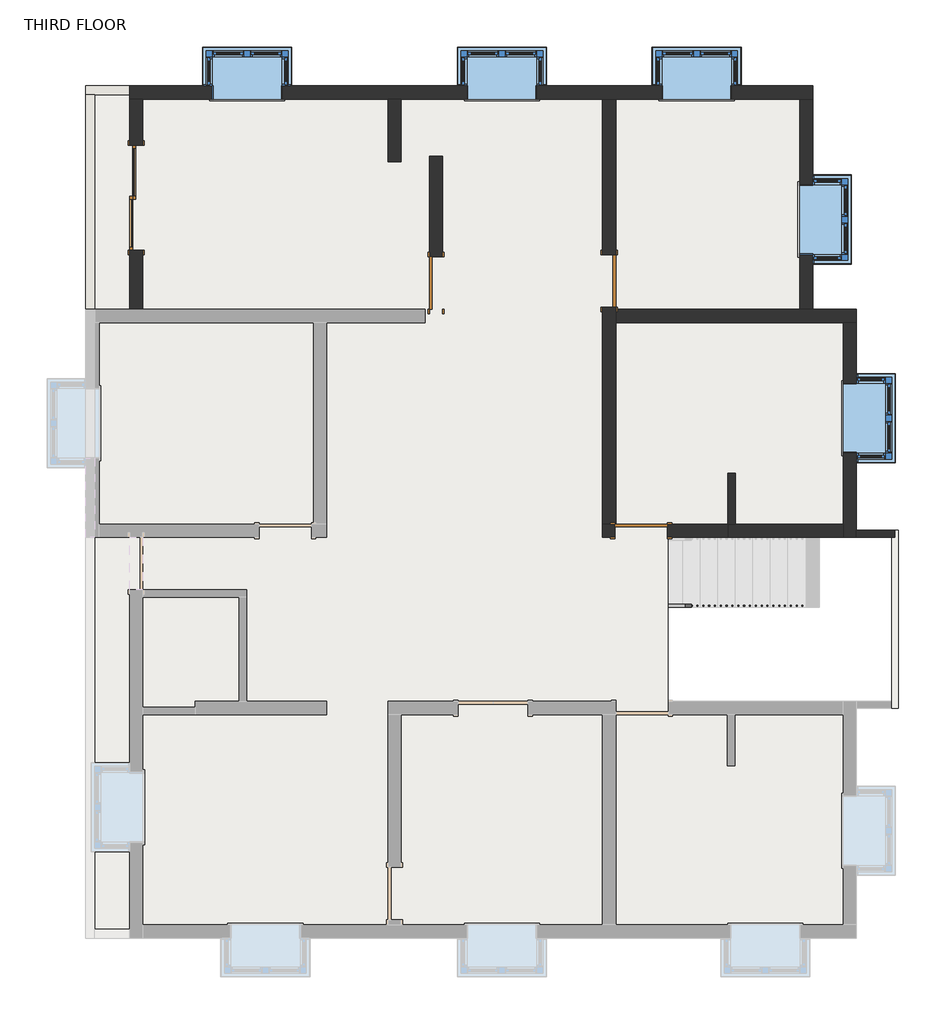
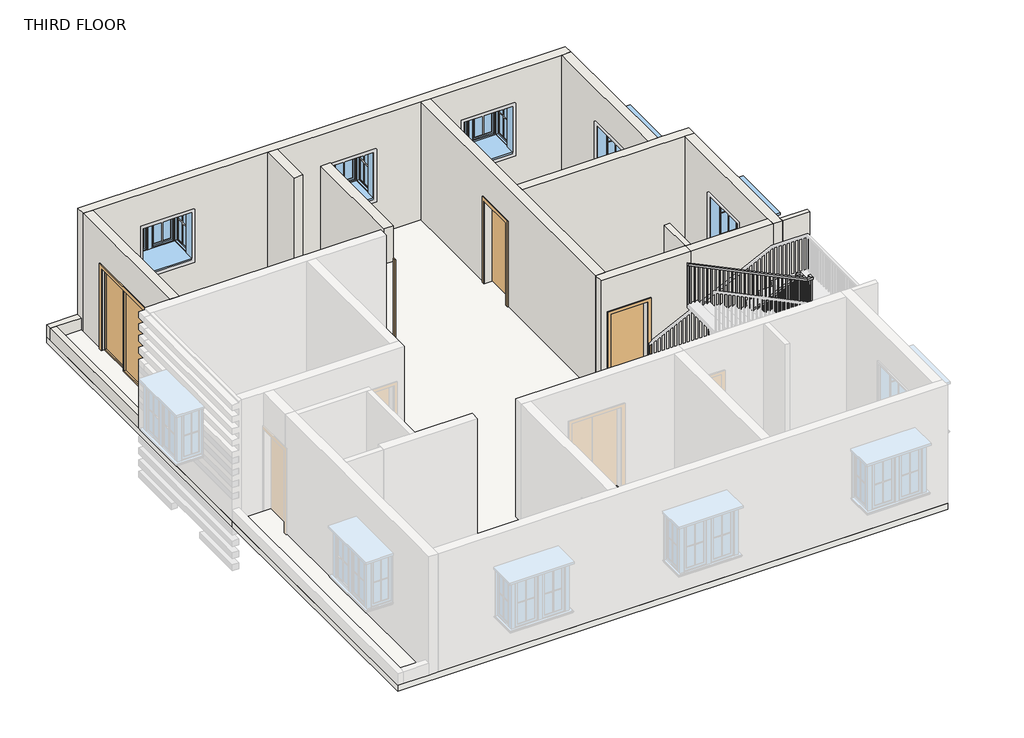
# One storey, part 2 of 4: 14 walls, 5 windows, 4 doors, 1 railing, 1 slab.
"""IFC4 building model written with IfcOpenShell, lengths in millimetres."""

from ifc_helpers import new_model, si_unit, frame, origin, place, context, project, spatial, polyline, outline, extrude, faceted_brep, transform, mapped, element, save
from components import door_d4d75d1e, door_a90ba1ad, door_0ca8825f, window_bay_casement_box_90_degree_angle_4_x4_x2_07b705a1

model = new_model("IFC4")

# Units and contexts
model_context = context("Model", 3, world=origin())
ifc_project = project(units=[si_unit("LENGTHUNIT", "METRE", prefix="MILLI")], contexts=[model_context])

# Site, building, storey
site = spatial("IfcSite", under=ifc_project)
building = spatial("IfcBuilding", under=site)
storey = spatial("IfcBuildingStorey", under=building, Name="THIRD FLOOR", Elevation=9601.2)

# Doors
placement = place(None, origin())
door_shape = door_d4d75d1e(model_context)
element("IfcDoor", 1, ObjectType="Door-Double-Sliding : 72\" x 84\"", at=placement, inside=storey, context=model_context, shape_type="MappedRepresentation", body=[
    mapped(door_shape, transform((-6005.0415084, 6126.233346, 9601.2), x_axis=(0.0, 1.0, 0.0), y_axis=(-1.0, 0.0, 0.0), z_axis=(0.0, 0.0, 1.0))),
])
door_2_shape = door_a90ba1ad(model_context)
element("IfcDoor", 2, ObjectType="Single-Flush : 36\" x 84\"", at=placement, inside=storey, context=model_context, shape_type="MappedRepresentation", body=[
    mapped(door_2_shape, transform((2656.3584916, 335.033346, 9601.2), x_axis=(-1.0, 0.0, 0.0), y_axis=(0.0, -1.0, 0.0), z_axis=(0.0, 0.0, 1.0))),
])
element("IfcDoor", 3, ObjectType="Single-Flush : 36\" x 84\"", at=placement, inside=storey, context=model_context, shape_type="MappedRepresentation", body=[
    mapped(door_2_shape, transform((-918.5024437, 4640.333346, 9601.2), x_axis=(0.0, -1.0, 0.0), y_axis=(1.0, 0.0, 0.0), z_axis=(0.0, 0.0, 1.0))),
])
door_3_shape = door_0ca8825f(model_context)
element("IfcDoor", 4, ObjectType="Single-Flush : 36\" x 84\"", at=placement, inside=storey, context=model_context, shape_type="MappedRepresentation", body=[
    mapped(door_3_shape, transform((2097.5584916, 4678.433346, 9601.2), x_axis=(0.0, -1.0, 0.0), y_axis=(1.0, 0.0, 0.0), z_axis=(0.0, 0.0, 1.0))),
])

# Railing
element("IfcRailing", 5, ObjectType="Handrail - Rectangular", at=placement, inside=storey, context=model_context, shape_type="SolidModel", body=[
    faceted_brep([(3126.2584916, -947.666654, 10661.0727273), (3126.2584916, -947.666654, 10604.5956113), (3126.2584916, -998.466654, 10604.5956113), (3126.2584916, -998.466654, 10661.0727273), (6044.5829507, -947.666654, 12078.7823634), (6095.3829507, -947.666654, 12046.9836718), (6095.3829507, -998.466654, 12046.9836718), (6044.5829507, -998.466654, 12078.7823634), (6044.5829507, -947.666654, 12115.8), (6095.3829507, -947.666654, 12065.0), (6095.3829507, -998.466654, 12065.0), (6044.5829507, -998.466654, 12115.8), (6171.5829507, -947.666654, 12115.8), (6171.5829507, -947.666654, 12065.0), (6120.7829507, -998.466654, 12065.0), (6120.7829507, -998.466654, 12115.8), (6171.5829507, -1074.666654, 12115.8), (6171.5829507, -1074.666654, 12065.0), (6120.7829507, -1074.666654, 12065.0), (6120.7829507, -1074.666654, 12115.8), (6171.5829507, -1341.366654, 12115.8), (6171.5829507, -1392.166654, 12065.0), (6120.7829507, -1392.166654, 12065.0), (6120.7829507, -1341.366654, 12115.8), (6171.5829507, -1341.366654, 12298.2903639), (6171.5829507, -1392.166654, 12247.4903639), (6120.7829507, -1392.166654, 12247.4903639), (6120.7829507, -1341.366654, 12298.2903639), (6171.5829507, -1468.366654, 12298.2903639), (6171.5829507, -1468.366654, 12247.4903639), (6120.7829507, -1417.566654, 12247.4903639), (6120.7829507, -1417.566654, 12298.2903639), (6044.5829507, -1468.366654, 12298.2903639), (6032.8967309, -1468.366654, 12247.4903639), (6032.8967309, -1417.566654, 12247.4903639), (6044.5829507, -1417.566654, 12298.2903639), (3126.2584916, -1468.366654, 13716.0), (3126.2584916, -1417.566654, 13716.0), (3126.2584916, -1417.566654, 13659.522884), (3126.2584916, -1468.366654, 13659.522884)], [[[0, 1, 2, 3]], [[1, 0, 4, 5]], [[2, 1, 5, 6]], [[3, 2, 6, 7]], [[0, 3, 7, 4]], [[5, 4, 8, 9]], [[6, 5, 9, 10]], [[7, 6, 10, 11]], [[4, 7, 11, 8]], [[9, 8, 12, 13]], [[10, 9, 13, 14]], [[11, 10, 14, 15]], [[8, 11, 15, 12]], [[13, 12, 16, 17]], [[14, 13, 17, 18]], [[15, 14, 18, 19]], [[12, 15, 19, 16]], [[17, 16, 20, 21]], [[18, 17, 21, 22]], [[19, 18, 22, 23]], [[16, 19, 23, 20]], [[21, 20, 24, 25]], [[22, 21, 25, 26]], [[23, 22, 26, 27]], [[20, 23, 27, 24]], [[25, 24, 28, 29]], [[26, 25, 29, 30]], [[27, 26, 30, 31]], [[24, 27, 31, 28]], [[29, 28, 32, 33]], [[30, 29, 33, 34]], [[31, 30, 34, 35]], [[28, 31, 35, 32]], [[36, 37, 38, 39]], [[33, 32, 36, 39]], [[34, 33, 39, 38]], [[35, 34, 38, 37]], [[32, 35, 37, 36]]]),
    extrude(outline(polyline([(13619.1778093, 3209.3079507), (13628.4322184, 3190.2579507), (12656.1272727, 3190.2579507), (12656.1272727, 3209.3079507), (13619.1778093, 3209.3079507)])), frame((0.0, -1452.491654, 0.0), z_axis=(0.0, 1.0, 0.0), x_axis=(0.0, 0.0, 1.0)), (0.0, 0.0, 1.0), 19.05),
    extrude(outline(polyline([(13569.8209605, 3310.9079507), (13579.0753696, 3291.8579507), (12656.1272727, 3291.8579507), (12656.1272727, 3310.9079507), (13569.8209605, 3310.9079507)])), frame((0.0, -1452.491654, 0.0), z_axis=(0.0, 1.0, 0.0), x_axis=(0.0, 0.0, 1.0)), (0.0, 0.0, 1.0), 19.05),
    extrude(outline(polyline([(13520.4641117, 3412.5079507), (13529.7185208, 3393.4579507), (12510.6545455, 3393.4579507), (12510.6545455, 3412.5079507), (13520.4641117, 3412.5079507)])), frame((0.0, -1452.491654, 0.0), z_axis=(0.0, 1.0, 0.0), x_axis=(0.0, 0.0, 1.0)), (0.0, 0.0, 1.0), 19.05),
    extrude(outline(polyline([(13471.1072629, 3514.1079507), (13480.3616721, 3495.0579507), (12510.6545455, 3495.0579507), (12510.6545455, 3514.1079507), (13471.1072629, 3514.1079507)])), frame((0.0, -1452.491654, 0.0), z_axis=(0.0, 1.0, 0.0), x_axis=(0.0, 0.0, 1.0)), (0.0, 0.0, 1.0), 19.05),
    extrude(outline(polyline([(13421.7504141, 3615.7079507), (13431.0048233, 3596.6579507), (12510.6545455, 3596.6579507), (12510.6545455, 3615.7079507), (13421.7504141, 3615.7079507)])), frame((0.0, -1452.491654, 0.0), z_axis=(0.0, 1.0, 0.0), x_axis=(0.0, 0.0, 1.0)), (0.0, 0.0, 1.0), 19.05),
    extrude(outline(polyline([(13372.3935653, 3717.3079507), (13381.6479745, 3698.2579507), (12365.1818182, 3698.2579507), (12365.1818182, 3717.3079507), (13372.3935653, 3717.3079507)])), frame((0.0, -1452.491654, 0.0), z_axis=(0.0, 1.0, 0.0), x_axis=(0.0, 0.0, 1.0)), (0.0, 0.0, 1.0), 19.05),
    extrude(outline(polyline([(13323.0367166, 3818.9079507), (13332.2911257, 3799.8579507), (12365.1818182, 3799.8579507), (12365.1818182, 3818.9079507), (13323.0367166, 3818.9079507)])), frame((0.0, -1452.491654, 0.0), z_axis=(0.0, 1.0, 0.0), x_axis=(0.0, 0.0, 1.0)), (0.0, 0.0, 1.0), 19.05),
    extrude(outline(polyline([(13273.6798678, 3920.5079507), (13282.9342769, 3901.4579507), (12365.1818182, 3901.4579507), (12365.1818182, 3920.5079507), (13273.6798678, 3920.5079507)])), frame((0.0, -1452.491654, 0.0), z_axis=(0.0, 1.0, 0.0), x_axis=(0.0, 0.0, 1.0)), (0.0, 0.0, 1.0), 19.05),
    extrude(outline(polyline([(13224.323019, 4022.1079507), (13233.5774281, 4003.0579507), (12219.7090909, 4003.0579507), (12219.7090909, 4022.1079507), (13224.323019, 4022.1079507)])), frame((0.0, -1452.491654, 0.0), z_axis=(0.0, 1.0, 0.0), x_axis=(0.0, 0.0, 1.0)), (0.0, 0.0, 1.0), 19.05),
    extrude(outline(polyline([(13174.9661702, 4123.7079507), (13184.2205793, 4104.6579507), (12219.7090909, 4104.6579507), (12219.7090909, 4123.7079507), (13174.9661702, 4123.7079507)])), frame((0.0, -1452.491654, 0.0), z_axis=(0.0, 1.0, 0.0), x_axis=(0.0, 0.0, 1.0)), (0.0, 0.0, 1.0), 19.05),
    extrude(outline(polyline([(13125.6093214, 4225.3079507), (13134.8637306, 4206.2579507), (12219.7090909, 4206.2579507), (12219.7090909, 4225.3079507), (13125.6093214, 4225.3079507)])), frame((0.0, -1452.491654, 0.0), z_axis=(0.0, 1.0, 0.0), x_axis=(0.0, 0.0, 1.0)), (0.0, 0.0, 1.0), 19.05),
    extrude(outline(polyline([(13076.2524726, 4326.9079507), (13085.5068818, 4307.8579507), (12074.2363636, 4307.8579507), (12074.2363636, 4326.9079507), (13076.2524726, 4326.9079507)])), frame((0.0, -1452.491654, 0.0), z_axis=(0.0, 1.0, 0.0), x_axis=(0.0, 0.0, 1.0)), (0.0, 0.0, 1.0), 19.05),
    extrude(outline(polyline([(13026.8956238, 4428.5079507), (13036.150033, 4409.4579507), (12074.2363636, 4409.4579507), (12074.2363636, 4428.5079507), (13026.8956238, 4428.5079507)])), frame((0.0, -1452.491654, 0.0), z_axis=(0.0, 1.0, 0.0), x_axis=(0.0, 0.0, 1.0)), (0.0, 0.0, 1.0), 19.05),
    extrude(outline(polyline([(12977.5387751, 4530.1079507), (12986.7931842, 4511.0579507), (12074.2363636, 4511.0579507), (12074.2363636, 4530.1079507), (12977.5387751, 4530.1079507)])), frame((0.0, -1452.491654, 0.0), z_axis=(0.0, 1.0, 0.0), x_axis=(0.0, 0.0, 1.0)), (0.0, 0.0, 1.0), 19.05),
    extrude(outline(polyline([(12928.1819263, 4631.7079507), (12937.4363354, 4612.6579507), (11928.7636364, 4612.6579507), (11928.7636364, 4631.7079507), (12928.1819263, 4631.7079507)])), frame((0.0, -1452.491654, 0.0), z_axis=(0.0, 1.0, 0.0), x_axis=(0.0, 0.0, 1.0)), (0.0, 0.0, 1.0), 19.05),
    extrude(outline(polyline([(12878.8250775, 4733.3079507), (12888.0794866, 4714.2579507), (11928.7636364, 4714.2579507), (11928.7636364, 4733.3079507), (12878.8250775, 4733.3079507)])), frame((0.0, -1452.491654, 0.0), z_axis=(0.0, 1.0, 0.0), x_axis=(0.0, 0.0, 1.0)), (0.0, 0.0, 1.0), 19.05),
    extrude(outline(polyline([(12829.4682287, 4834.9079507), (12838.7226379, 4815.8579507), (11928.7636364, 4815.8579507), (11928.7636364, 4834.9079507), (12829.4682287, 4834.9079507)])), frame((0.0, -1452.491654, 0.0), z_axis=(0.0, 1.0, 0.0), x_axis=(0.0, 0.0, 1.0)), (0.0, 0.0, 1.0), 19.05),
    extrude(outline(polyline([(12780.1113799, 4936.5079507), (12789.3657891, 4917.4579507), (11783.2909091, 4917.4579507), (11783.2909091, 4936.5079507), (12780.1113799, 4936.5079507)])), frame((0.0, -1452.491654, 0.0), z_axis=(0.0, 1.0, 0.0), x_axis=(0.0, 0.0, 1.0)), (0.0, 0.0, 1.0), 19.05),
    extrude(outline(polyline([(12730.7545311, 5038.1079507), (12740.0089403, 5019.0579507), (11783.2909091, 5019.0579507), (11783.2909091, 5038.1079507), (12730.7545311, 5038.1079507)])), frame((0.0, -1452.491654, 0.0), z_axis=(0.0, 1.0, 0.0), x_axis=(0.0, 0.0, 1.0)), (0.0, 0.0, 1.0), 19.05),
    extrude(outline(polyline([(12681.3976824, 5139.7079507), (12690.6520915, 5120.6579507), (11783.2909091, 5120.6579507), (11783.2909091, 5139.7079507), (12681.3976824, 5139.7079507)])), frame((0.0, -1452.491654, 0.0), z_axis=(0.0, 1.0, 0.0), x_axis=(0.0, 0.0, 1.0)), (0.0, 0.0, 1.0), 19.05),
    extrude(outline(polyline([(12631.959384, 5241.3079507), (12641.2137931, 5222.2579507), (11637.8181818, 5222.2579507), (11637.8181818, 5241.3079507), (12631.959384, 5241.3079507)])), frame((0.0, -1452.491654, 0.0), z_axis=(0.0, 1.0, 0.0), x_axis=(0.0, 0.0, 1.0)), (0.0, 0.0, 1.0), 19.05),
    extrude(outline(polyline([(12582.6839848, 5342.9079507), (12591.9383939, 5323.8579507), (11637.8181818, 5323.8579507), (11637.8181818, 5342.9079507), (12582.6839848, 5342.9079507)])), frame((0.0, -1452.491654, 0.0), z_axis=(0.0, 1.0, 0.0), x_axis=(0.0, 0.0, 1.0)), (0.0, 0.0, 1.0), 19.05),
    extrude(outline(polyline([(12533.327136, 5444.5079507), (12542.5815452, 5425.4579507), (11637.8181818, 5425.4579507), (11637.8181818, 5444.5079507), (12533.327136, 5444.5079507)])), frame((0.0, -1452.491654, 0.0), z_axis=(0.0, 1.0, 0.0), x_axis=(0.0, 0.0, 1.0)), (0.0, 0.0, 1.0), 19.05),
    extrude(outline(polyline([(12483.9702872, 5546.1079507), (12493.2246964, 5527.0579507), (11492.3454545, 5527.0579507), (11492.3454545, 5546.1079507), (12483.9702872, 5546.1079507)])), frame((0.0, -1452.491654, 0.0), z_axis=(0.0, 1.0, 0.0), x_axis=(0.0, 0.0, 1.0)), (0.0, 0.0, 1.0), 19.05),
    extrude(outline(polyline([(12434.6134384, 5647.7079507), (12443.8678476, 5628.6579507), (11492.3454545, 5628.6579507), (11492.3454545, 5647.7079507), (12434.6134384, 5647.7079507)])), frame((0.0, -1452.491654, 0.0), z_axis=(0.0, 1.0, 0.0), x_axis=(0.0, 0.0, 1.0)), (0.0, 0.0, 1.0), 19.05),
    extrude(outline(polyline([(12385.2565897, 5749.3079507), (12394.5109988, 5730.2579507), (11492.3454545, 5730.2579507), (11492.3454545, 5749.3079507), (12385.2565897, 5749.3079507)])), frame((0.0, -1452.491654, 0.0), z_axis=(0.0, 1.0, 0.0), x_axis=(0.0, 0.0, 1.0)), (0.0, 0.0, 1.0), 19.05),
    extrude(outline(polyline([(12335.8997409, 5850.9079507), (12345.15415, 5831.8579507), (11346.8727273, 5831.8579507), (11346.8727273, 5850.9079507), (12335.8997409, 5850.9079507)])), frame((0.0, -1452.491654, 0.0), z_axis=(0.0, 1.0, 0.0), x_axis=(0.0, 0.0, 1.0)), (0.0, 0.0, 1.0), 19.05),
    extrude(outline(polyline([(12286.5428921, 5952.5079507), (12295.7973012, 5933.4579507), (11346.8727273, 5933.4579507), (11346.8727273, 5952.5079507), (12286.5428921, 5952.5079507)])), frame((0.0, -1452.491654, 0.0), z_axis=(0.0, 1.0, 0.0), x_axis=(0.0, 0.0, 1.0)), (0.0, 0.0, 1.0), 19.05),
    extrude(outline(polyline([(12237.1860433, 6054.1079507), (12246.4404524, 6035.0579507), (11346.8727273, 6035.0579507), (11346.8727273, 6054.1079507), (12237.1860433, 6054.1079507)])), frame((0.0, -1452.491654, 0.0), z_axis=(0.0, 1.0, 0.0), x_axis=(0.0, 0.0, 1.0)), (0.0, 0.0, 1.0), 19.05),
    extrude(outline(polyline([(6136.6579507, -1369.941654), (6155.7079507, -1369.941654), (6155.7079507, -1388.991654), (6136.6579507, -1388.991654), (6136.6579507, -1369.941654)])), frame((0.0, 0.0, 11201.4), z_axis=(0.0, 0.0, 1.0), x_axis=(1.0, 0.0, 0.0)), (0.0, 0.0, 1.0), 1046.0903639),
    extrude(outline(polyline([(6136.6579507, -1268.341654), (6155.7079507, -1268.341654), (6155.7079507, -1287.391654), (6136.6579507, -1287.391654), (6136.6579507, -1268.341654)])), frame((0.0, 0.0, 11201.4), z_axis=(0.0, 0.0, 1.0), x_axis=(1.0, 0.0, 0.0)), (0.0, 0.0, 1.0), 863.6),
    extrude(outline(polyline([(6136.6579507, -1166.741654), (6155.7079507, -1166.741654), (6155.7079507, -1185.791654), (6136.6579507, -1185.791654), (6136.6579507, -1166.741654)])), frame((0.0, 0.0, 11201.4), z_axis=(0.0, 0.0, 1.0), x_axis=(1.0, 0.0, 0.0)), (0.0, 0.0, 1.0), 863.6),
    extrude(outline(polyline([(6136.6579507, -1065.141654), (6155.7079507, -1065.141654), (6155.7079507, -1084.191654), (6136.6579507, -1084.191654), (6136.6579507, -1065.141654)])), frame((0.0, 0.0, 11201.4), z_axis=(0.0, 0.0, 1.0), x_axis=(1.0, 0.0, 0.0)), (0.0, 0.0, 1.0), 863.6),
    extrude(outline(polyline([(6063.1334916, -982.591654), (6063.1334916, -963.541654), (6082.1834916, -963.541654), (6082.1834916, -982.591654), (6063.1334916, -982.591654)])), frame((0.0, 0.0, 11055.9272727), z_axis=(0.0, 0.0, 1.0), x_axis=(1.0, 0.0, 0.0)), (0.0, 0.0, 1.0), 1009.0727273),
    extrude(outline(polyline([(11991.2145818, 5980.5834916), (11981.9601727, 5961.5334916), (11055.9272727, 5961.5334916), (11055.9272727, 5980.5834916), (11991.2145818, 5980.5834916)])), frame((0.0, -982.591654, 0.0), z_axis=(0.0, 1.0, 0.0), x_axis=(0.0, 0.0, 1.0)), (0.0, 0.0, 1.0), 19.05),
    extrude(outline(polyline([(11941.857733, 5878.9834916), (11932.6033239, 5859.9334916), (11055.9272727, 5859.9334916), (11055.9272727, 5878.9834916), (11941.857733, 5878.9834916)])), frame((0.0, -982.591654, 0.0), z_axis=(0.0, 1.0, 0.0), x_axis=(0.0, 0.0, 1.0)), (0.0, 0.0, 1.0), 19.05),
    extrude(outline(polyline([(11892.5008843, 5777.3834916), (11883.2464751, 5758.3334916), (10910.4545455, 5758.3334916), (10910.4545455, 5777.3834916), (11892.5008843, 5777.3834916)])), frame((0.0, -982.591654, 0.0), z_axis=(0.0, 1.0, 0.0), x_axis=(0.0, 0.0, 1.0)), (0.0, 0.0, 1.0), 19.05),
    extrude(outline(polyline([(11843.1440355, 5675.7834916), (11833.8896263, 5656.7334916), (10910.4545455, 5656.7334916), (10910.4545455, 5675.7834916), (11843.1440355, 5675.7834916)])), frame((0.0, -982.591654, 0.0), z_axis=(0.0, 1.0, 0.0), x_axis=(0.0, 0.0, 1.0)), (0.0, 0.0, 1.0), 19.05),
    extrude(outline(polyline([(11793.7871867, 5574.1834916), (11784.5327775, 5555.1334916), (10910.4545455, 5555.1334916), (10910.4545455, 5574.1834916), (11793.7871867, 5574.1834916)])), frame((0.0, -982.591654, 0.0), z_axis=(0.0, 1.0, 0.0), x_axis=(0.0, 0.0, 1.0)), (0.0, 0.0, 1.0), 19.05),
    extrude(outline(polyline([(11744.4303379, 5472.5834916), (11735.1759288, 5453.5334916), (10764.9818182, 5453.5334916), (10764.9818182, 5472.5834916), (11744.4303379, 5472.5834916)])), frame((0.0, -982.591654, 0.0), z_axis=(0.0, 1.0, 0.0), x_axis=(0.0, 0.0, 1.0)), (0.0, 0.0, 1.0), 19.05),
    extrude(outline(polyline([(11695.0734891, 5370.9834916), (11685.81908, 5351.9334916), (10764.9818182, 5351.9334916), (10764.9818182, 5370.9834916), (11695.0734891, 5370.9834916)])), frame((0.0, -982.591654, 0.0), z_axis=(0.0, 1.0, 0.0), x_axis=(0.0, 0.0, 1.0)), (0.0, 0.0, 1.0), 19.05),
    extrude(outline(polyline([(11645.7166403, 5269.3834916), (11636.4622312, 5250.3334916), (10764.9818182, 5250.3334916), (10764.9818182, 5269.3834916), (11645.7166403, 5269.3834916)])), frame((0.0, -982.591654, 0.0), z_axis=(0.0, 1.0, 0.0), x_axis=(0.0, 0.0, 1.0)), (0.0, 0.0, 1.0), 19.05),
    extrude(outline(polyline([(11596.3597915, 5167.7834916), (11587.1053824, 5148.7334916), (10619.5090909, 5148.7334916), (10619.5090909, 5167.7834916), (11596.3597915, 5167.7834916)])), frame((0.0, -982.591654, 0.0), z_axis=(0.0, 1.0, 0.0), x_axis=(0.0, 0.0, 1.0)), (0.0, 0.0, 1.0), 19.05),
    extrude(outline(polyline([(11547.0029428, 5066.1834916), (11537.7485336, 5047.1334916), (10619.5090909, 5047.1334916), (10619.5090909, 5066.1834916), (11547.0029428, 5066.1834916)])), frame((0.0, -982.591654, 0.0), z_axis=(0.0, 1.0, 0.0), x_axis=(0.0, 0.0, 1.0)), (0.0, 0.0, 1.0), 19.05),
    extrude(outline(polyline([(11497.646094, 4964.5834916), (11488.3916848, 4945.5334916), (10619.5090909, 4945.5334916), (10619.5090909, 4964.5834916), (11497.646094, 4964.5834916)])), frame((0.0, -982.591654, 0.0), z_axis=(0.0, 1.0, 0.0), x_axis=(0.0, 0.0, 1.0)), (0.0, 0.0, 1.0), 19.05),
    extrude(outline(polyline([(11448.2892452, 4862.9834916), (11439.034836, 4843.9334916), (10474.0363636, 4843.9334916), (10474.0363636, 4862.9834916), (11448.2892452, 4862.9834916)])), frame((0.0, -982.591654, 0.0), z_axis=(0.0, 1.0, 0.0), x_axis=(0.0, 0.0, 1.0)), (0.0, 0.0, 1.0), 19.05),
    extrude(outline(polyline([(11398.9323964, 4761.3834916), (11389.6779873, 4742.3334916), (10474.0363636, 4742.3334916), (10474.0363636, 4761.3834916), (11398.9323964, 4761.3834916)])), frame((0.0, -982.591654, 0.0), z_axis=(0.0, 1.0, 0.0), x_axis=(0.0, 0.0, 1.0)), (0.0, 0.0, 1.0), 19.05),
    extrude(outline(polyline([(11349.5755476, 4659.7834916), (11340.3211385, 4640.7334916), (10474.0363636, 4640.7334916), (10474.0363636, 4659.7834916), (11349.5755476, 4659.7834916)])), frame((0.0, -982.591654, 0.0), z_axis=(0.0, 1.0, 0.0), x_axis=(0.0, 0.0, 1.0)), (0.0, 0.0, 1.0), 19.05),
    extrude(outline(polyline([(11300.2186988, 4558.1834916), (11290.9642897, 4539.1334916), (10328.5636364, 4539.1334916), (10328.5636364, 4558.1834916), (11300.2186988, 4558.1834916)])), frame((0.0, -982.591654, 0.0), z_axis=(0.0, 1.0, 0.0), x_axis=(0.0, 0.0, 1.0)), (0.0, 0.0, 1.0), 19.05),
    extrude(outline(polyline([(11250.8618501, 4456.5834916), (11241.6074409, 4437.5334916), (10328.5636364, 4437.5334916), (10328.5636364, 4456.5834916), (11250.8618501, 4456.5834916)])), frame((0.0, -982.591654, 0.0), z_axis=(0.0, 1.0, 0.0), x_axis=(0.0, 0.0, 1.0)), (0.0, 0.0, 1.0), 19.05),
    extrude(outline(polyline([(11201.5050013, 4354.9834916), (11192.2505921, 4335.9334916), (10328.5636364, 4335.9334916), (10328.5636364, 4354.9834916), (11201.5050013, 4354.9834916)])), frame((0.0, -982.591654, 0.0), z_axis=(0.0, 1.0, 0.0), x_axis=(0.0, 0.0, 1.0)), (0.0, 0.0, 1.0), 19.05),
    extrude(outline(polyline([(11152.1481525, 4253.3834916), (11142.8937433, 4234.3334916), (10183.0909091, 4234.3334916), (10183.0909091, 4253.3834916), (11152.1481525, 4253.3834916)])), frame((0.0, -982.591654, 0.0), z_axis=(0.0, 1.0, 0.0), x_axis=(0.0, 0.0, 1.0)), (0.0, 0.0, 1.0), 19.05),
    extrude(outline(polyline([(11102.7913037, 4151.7834916), (11093.5368946, 4132.7334916), (10183.0909091, 4132.7334916), (10183.0909091, 4151.7834916), (11102.7913037, 4151.7834916)])), frame((0.0, -982.591654, 0.0), z_axis=(0.0, 1.0, 0.0), x_axis=(0.0, 0.0, 1.0)), (0.0, 0.0, 1.0), 19.05),
    extrude(outline(polyline([(11053.4344549, 4050.1834916), (11044.1800458, 4031.1334916), (10183.0909091, 4031.1334916), (10183.0909091, 4050.1834916), (11053.4344549, 4050.1834916)])), frame((0.0, -982.591654, 0.0), z_axis=(0.0, 1.0, 0.0), x_axis=(0.0, 0.0, 1.0)), (0.0, 0.0, 1.0), 19.05),
    extrude(outline(polyline([(11004.0776061, 3948.5834916), (10994.823197, 3929.5334916), (10037.6181818, 3929.5334916), (10037.6181818, 3948.5834916), (11004.0776061, 3948.5834916)])), frame((0.0, -982.591654, 0.0), z_axis=(0.0, 1.0, 0.0), x_axis=(0.0, 0.0, 1.0)), (0.0, 0.0, 1.0), 19.05),
    extrude(outline(polyline([(10954.7207573, 3846.9834916), (10945.4663482, 3827.9334916), (10037.6181818, 3827.9334916), (10037.6181818, 3846.9834916), (10954.7207573, 3846.9834916)])), frame((0.0, -982.591654, 0.0), z_axis=(0.0, 1.0, 0.0), x_axis=(0.0, 0.0, 1.0)), (0.0, 0.0, 1.0), 19.05),
    extrude(outline(polyline([(10905.3639086, 3745.3834916), (10896.1094994, 3726.3334916), (10037.6181818, 3726.3334916), (10037.6181818, 3745.3834916), (10905.3639086, 3745.3834916)])), frame((0.0, -982.591654, 0.0), z_axis=(0.0, 1.0, 0.0), x_axis=(0.0, 0.0, 1.0)), (0.0, 0.0, 1.0), 19.05),
    extrude(outline(polyline([(10856.0070598, 3643.7834916), (10846.7526506, 3624.7334916), (9892.1454545, 3624.7334916), (9892.1454545, 3643.7834916), (10856.0070598, 3643.7834916)])), frame((0.0, -982.591654, 0.0), z_axis=(0.0, 1.0, 0.0), x_axis=(0.0, 0.0, 1.0)), (0.0, 0.0, 1.0), 19.05),
    extrude(outline(polyline([(10806.650211, 3542.1834916), (10797.3958018, 3523.1334916), (9892.1454545, 3523.1334916), (9892.1454545, 3542.1834916), (10806.650211, 3542.1834916)])), frame((0.0, -982.591654, 0.0), z_axis=(0.0, 1.0, 0.0), x_axis=(0.0, 0.0, 1.0)), (0.0, 0.0, 1.0), 19.05),
    extrude(outline(polyline([(10757.2933622, 3440.5834916), (10748.0389531, 3421.5334916), (9892.1454545, 3421.5334916), (9892.1454545, 3440.5834916), (10757.2933622, 3440.5834916)])), frame((0.0, -982.591654, 0.0), z_axis=(0.0, 1.0, 0.0), x_axis=(0.0, 0.0, 1.0)), (0.0, 0.0, 1.0), 19.05),
    extrude(outline(polyline([(10707.9365134, 3338.9834916), (10698.6821043, 3319.9334916), (9746.6727273, 3319.9334916), (9746.6727273, 3338.9834916), (10707.9365134, 3338.9834916)])), frame((0.0, -982.591654, 0.0), z_axis=(0.0, 1.0, 0.0), x_axis=(0.0, 0.0, 1.0)), (0.0, 0.0, 1.0), 19.05),
    extrude(outline(polyline([(10658.5796646, 3237.3834916), (10649.3252555, 3218.3334916), (9746.6727273, 3218.3334916), (9746.6727273, 3237.3834916), (10658.5796646, 3237.3834916)])), frame((0.0, -982.591654, 0.0), z_axis=(0.0, 1.0, 0.0), x_axis=(0.0, 0.0, 1.0)), (0.0, 0.0, 1.0), 19.05),
    extrude(outline(polyline([(6136.6579507, -1433.441654), (6155.7079507, -1433.441654), (6155.7079507, -1452.491654), (6136.6579507, -1452.491654), (6136.6579507, -1433.441654)])), frame((0.0, 0.0, 11201.4), z_axis=(0.0, 0.0, 1.0), x_axis=(1.0, 0.0, 0.0)), (0.0, 0.0, 1.0), 1046.0903639),
    extrude(outline(polyline([(6136.6579507, -982.591654), (6136.6579507, -963.541654), (6155.7079507, -963.541654), (6155.7079507, -982.591654), (6136.6579507, -982.591654)])), frame((0.0, 0.0, 11201.4), z_axis=(0.0, 0.0, 1.0), x_axis=(1.0, 0.0, 0.0)), (0.0, 0.0, 1.0), 863.6),
    extrude(outline(polyline([(13650.2684749, 3145.3084916), (13659.522884, 3126.2584916), (12656.1272727, 3126.2584916), (12656.1272727, 3145.3084916), (13650.2684749, 3145.3084916)])), frame((0.0, -1452.491654, 0.0), z_axis=(0.0, 1.0, 0.0), x_axis=(0.0, 0.0, 1.0)), (0.0, 0.0, 1.0), 19.05),
    extrude(outline(polyline([(10613.8500204, 3145.3084916), (10604.5956113, 3126.2584916), (9746.6727273, 3126.2584916), (9746.6727273, 3145.3084916), (10613.8500204, 3145.3084916)])), frame((0.0, -982.591654, 0.0), z_axis=(0.0, 1.0, 0.0), x_axis=(0.0, 0.0, 1.0)), (0.0, 0.0, 1.0), 19.05),
])

# Slab
element("IfcSlab", 6, ObjectType="6\"", at=placement, inside=storey, context=model_context, shape_type="SweptSolid", body=[
    extrude(outline(polyline([(-7008.3415084, -6751.566654), (-7008.3415084, 220.733346), (-7008.3415084, 8069.333346), (5640.8584916, 8069.333346), (5640.8584916, 4183.133346), (6402.8584916, 4183.133346), (6402.8584916, 337.573346), (7125.9750459, 337.573346), (7125.9750459, -2753.606654), (6402.8584916, -2753.606654), (6402.8584916, -6751.566654), (-7008.3415084, -6751.566654)]), holes=[polyline([(7009.1350459, 220.733346), (3126.2584916, 220.733346), (3126.2584916, -2636.766654), (7009.1350459, -2636.766654), (7009.1350459, 220.733346)])]), frame((0.0, 0.0, 9448.8), z_axis=(0.0, 0.0, 1.0), x_axis=(1.0, 0.0, 0.0)), (0.0, 0.0, 1.0), 152.4),
])

# Walls
element("IfcWall", 7, ObjectType="4.6\"", at=placement, inside=storey, context=model_context, shape_type="SweptSolid", body=[
    extrude(outline(polyline([(7067.5550459, 220.733346), (6402.8584916, 220.733346), (6402.8584916, 337.573346), (7067.5550459, 337.573346), (7067.5550459, 220.733346)])), frame((0.0, 0.0, 9601.2), z_axis=(0.0, 0.0, 1.0), x_axis=(1.0, 0.0, 0.0)), (0.0, 0.0, 1.0), 3048.0),
])
element("IfcWall", 8, ObjectType="5\"", at=placement, inside=storey, context=model_context, shape_type="SweptSolid", body=[
    extrude(outline(polyline([(4291.9829507, 1335.1417393), (4291.9829507, 449.333346), (4164.9829507, 449.333346), (4164.9829507, 1335.1417393), (4291.9829507, 1335.1417393)])), frame((0.0, 0.0, 9601.2), z_axis=(0.0, 0.0, 1.0), x_axis=(1.0, 0.0, 0.0)), (0.0, 0.0, 1.0), 3048.0),
])
element("IfcWall", 9, ObjectType="6\"", at=placement, inside=storey, context=model_context, shape_type="Brep", body=[
    faceted_brep([(-6246.3415084, 8069.333346, 9601.2), (-7008.3415084, 8069.333346, 9601.2), (-7008.3415084, 8069.333346, 9906.0), (-6246.3415084, 8069.333346, 9906.0), (-6246.3415084, 7916.933346, 9601.2), (-6246.3415084, 7916.933346, 9906.0), (-6855.9415084, 7916.933346, 9906.0), (-7008.3415084, 7916.933346, 9906.0), (-7008.3415084, 7916.933346, 9601.2), (-6855.9415084, 7916.933346, 9601.2)], [[[0, 1, 2, 3]], [[4, 5, 6, 7, 8, 9]], [[1, 0, 4, 9, 8]], [[3, 2, 7, 6, 5]], [[2, 1, 8, 7]], [[0, 3, 5, 4]]]),
])
element("IfcWall", 10, ObjectType="6\"", at=placement, inside=storey, context=model_context, shape_type="SweptSolid", body=[
    extrude(outline(polyline([(-7008.3415084, 4183.133346), (-7008.3415084, 7916.933346), (-6855.9415084, 7916.933346), (-6855.9415084, 4183.133346), (-7008.3415084, 4183.133346)])), frame((0.0, 0.0, 9601.2), z_axis=(0.0, 0.0, 1.0), x_axis=(1.0, 0.0, 0.0)), (0.0, 0.0, 1.0), 304.8),
])
element("IfcWall", 11, ObjectType="9\"", at=placement, inside=storey, context=model_context, shape_type="Brep", body=[
    faceted_brep([(5640.8584916, 8069.333346, 9601.2), (-6246.3415084, 8069.333346, 9601.2), (-6246.3415084, 8069.333346, 9906.0), (-6246.3415084, 8069.333346, 12649.2), (5640.8584916, 8069.333346, 12649.2), (-3592.0415084, 8069.333346, 11785.6), (-4811.2415084, 8069.333346, 11785.6), (-4811.2415084, 8069.333346, 10515.6), (-3592.0415084, 8069.333346, 10515.6), (4231.1584916, 8069.333346, 11785.6), (3011.9584916, 8069.333346, 11785.6), (3011.9584916, 8069.333346, 10515.6), (4231.1584916, 8069.333346, 10515.6), (840.2584916, 8069.333346, 11785.6), (-378.9415084, 8069.333346, 11785.6), (-378.9415084, 8069.333346, 10515.6), (840.2584916, 8069.333346, 10515.6), (5640.8584916, 7840.733346, 9601.2), (5640.8584916, 7840.733346, 12649.2), (5412.2584916, 7840.733346, 12649.2), (2211.8584916, 7840.733346, 12649.2), (1983.2584916, 7840.733346, 12649.2), (-1521.9415084, 7840.733346, 12649.2), (-1750.5415084, 7840.733346, 12649.2), (-6017.7415084, 7840.733346, 12649.2), (-6246.3415084, 7840.733346, 12649.2), (-6246.3415084, 7840.733346, 9601.2), (-6017.7415084, 7840.733346, 9601.2), (-1750.5415084, 7840.733346, 9601.2), (-1521.9415084, 7840.733346, 9601.2), (1983.2584916, 7840.733346, 9601.2), (2211.8584916, 7840.733346, 9601.2), (5412.2584916, 7840.733346, 9601.2), (-3592.0415084, 7840.733346, 11785.6), (-3592.0415084, 7840.733346, 10515.6), (-4811.2415084, 7840.733346, 10515.6), (-4811.2415084, 7840.733346, 11785.6), (4231.1584916, 7840.733346, 11785.6), (4231.1584916, 7840.733346, 10515.6), (3011.9584916, 7840.733346, 10515.6), (3011.9584916, 7840.733346, 11785.6), (840.2584916, 7840.733346, 11785.6), (840.2584916, 7840.733346, 10515.6), (-378.9415084, 7840.733346, 10515.6), (-378.9415084, 7840.733346, 11785.6), (-6246.3415084, 7916.933346, 9601.2)], [[[0, 1, 2, 3, 4], [5, 6, 7, 8], [9, 10, 11, 12], [13, 14, 15, 16]], [[17, 18, 19, 20, 21, 22, 23, 24, 25, 26, 27, 28, 29, 30, 31, 32], [33, 34, 35, 36], [37, 38, 39, 40], [41, 42, 43, 44]], [[1, 0, 17, 32, 31, 30, 29, 28, 27, 26, 45]], [[4, 3, 25, 24, 23, 22, 21, 20, 19, 18]], [[0, 4, 18, 17]], [[34, 33, 5, 8]], [[35, 34, 8, 7]], [[36, 35, 7, 6]], [[33, 36, 6, 5]], [[38, 37, 9, 12]], [[39, 38, 12, 11]], [[40, 39, 11, 10]], [[37, 40, 10, 9]], [[42, 41, 13, 16]], [[43, 42, 16, 15]], [[44, 43, 15, 14]], [[41, 44, 14, 13]], [[1, 45, 26, 25, 3, 2]]]),
])
element("IfcWall", 12, ObjectType="9\"", at=placement, inside=storey, context=model_context, shape_type="SweptSolid", body=[
    extrude(outline(polyline([(7840.733346, 9601.2), (7040.633346, 9601.2), (7040.633346, 11734.8), (5211.833346, 11734.8), (5211.833346, 9601.2), (4183.133346, 9601.2), (4183.133346, 12649.2), (7840.733346, 12649.2), (7840.733346, 9601.2)])), frame((-6246.3415084, 0.0, 0.0), z_axis=(1.0, 0.0, 0.0), x_axis=(0.0, 1.0, 0.0)), (0.0, 0.0, 1.0), 228.6),
])
element("IfcWall", 13, ObjectType="9\"", at=placement, inside=storey, context=model_context, shape_type="SweptSolid", body=[
    extrude(outline(polyline([(7840.733346, 9601.2), (4183.133346, 9601.2), (4183.133346, 12649.2), (7840.733346, 12649.2), (7840.733346, 9601.2)]), holes=[polyline([(5135.633346, 11785.6), (5135.633346, 10515.6), (6354.833346, 10515.6), (6354.833346, 11785.6), (5135.633346, 11785.6)])]), frame((5412.2584916, 0.0, 0.0), z_axis=(1.0, 0.0, 0.0), x_axis=(0.0, 1.0, 0.0)), (0.0, 0.0, 1.0), 228.6),
])
element("IfcWall", 14, ObjectType="9\"", at=placement, inside=storey, context=model_context, shape_type="Brep", body=[
    faceted_brep([(1983.2584916, 4221.233346, 11734.8), (1983.2584916, 4221.233346, 9601.2), (1983.2584916, 449.333346, 9601.2), (1983.2584916, 449.333346, 12649.2), (1983.2584916, 7840.733346, 12649.2), (1983.2584916, 7840.733346, 9601.2), (1983.2584916, 5135.633346, 9601.2), (1983.2584916, 5135.633346, 11734.8), (2211.8584916, 449.333346, 9601.2), (2211.8584916, 3954.533346, 9601.2), (2211.8584916, 4183.133346, 9601.2), (2211.8584916, 4221.233346, 9601.2), (2211.8584916, 4221.233346, 11734.8), (2211.8584916, 5135.633346, 11734.8), (2211.8584916, 5135.633346, 9601.2), (2211.8584916, 7840.733346, 9601.2), (2211.8584916, 7840.733346, 12649.2), (2211.8584916, 4183.133346, 12649.2), (2211.8584916, 3954.533346, 12649.2), (2211.8584916, 449.333346, 12649.2), (2199.1584916, 449.333346, 9601.2)], [[[0, 1, 2, 3, 4, 5, 6, 7]], [[8, 9, 10, 11, 12, 13, 14, 15, 16, 17, 18, 19]], [[6, 5, 15, 14]], [[2, 1, 11, 10, 9, 8, 20]], [[4, 3, 19, 18, 17, 16]], [[5, 4, 16, 15]], [[3, 2, 20, 8, 19]], [[12, 11, 1, 0]], [[13, 12, 0, 7]], [[14, 13, 7, 6]]]),
])
element("IfcWall", 15, ObjectType="9\"", at=placement, inside=storey, context=model_context, shape_type="SweptSolid", body=[
    extrude(outline(polyline([(-1750.5415084, 6747.0175593), (-1750.5415084, 7840.733346), (-1521.9415084, 7840.733346), (-1521.9415084, 6747.0175593), (-1750.5415084, 6747.0175593)])), frame((0.0, 0.0, 9601.2), z_axis=(0.0, 0.0, 1.0), x_axis=(1.0, 0.0, 0.0)), (0.0, 0.0, 1.0), 3048.0),
])
element("IfcWall", 16, ObjectType="9\"", at=placement, inside=storey, context=model_context, shape_type="Brep", body=[
    faceted_brep([(6402.8584916, 4183.133346, 9601.2), (5640.8584916, 4183.133346, 9601.2), (5412.2584916, 4183.133346, 9601.2), (2211.8584916, 4183.133346, 9601.2), (2211.8584916, 4183.133346, 12649.2), (5412.2584916, 4183.133346, 12649.2), (5640.8584916, 4183.133346, 12649.2), (6402.8584916, 4183.133346, 12649.2), (6402.8584916, 3954.533346, 9601.2), (6402.8584916, 3954.533346, 12649.2), (6174.2584916, 3954.533346, 12649.2), (2211.8584916, 3954.533346, 12649.2), (2211.8584916, 3954.533346, 9601.2), (6174.2584916, 3954.533346, 9601.2)], [[[0, 1, 2, 3, 4, 5, 6, 7]], [[8, 9, 10, 11, 12, 13]], [[3, 2, 1, 0, 8, 13, 12]], [[7, 6, 5, 4, 11, 10, 9]], [[4, 3, 12, 11]], [[0, 7, 9, 8]]]),
])
element("IfcWall", 17, ObjectType="9\"", at=placement, inside=storey, context=model_context, shape_type="Brep", body=[
    faceted_brep([(6174.2584916, 3954.533346, 9601.2), (6174.2584916, 449.333346, 9601.2), (6174.2584916, 220.733346, 9601.2), (6174.2584916, 220.733346, 12649.2), (6174.2584916, 449.333346, 12649.2), (6174.2584916, 3954.533346, 12649.2), (6174.2584916, 1681.233346, 11785.6), (6174.2584916, 1681.233346, 10515.6), (6174.2584916, 2900.433346, 10515.6), (6174.2584916, 2900.433346, 11785.6), (6402.8584916, 3954.533346, 9601.2), (6402.8584916, 3954.533346, 12649.2), (6402.8584916, 337.573346, 12649.2), (6402.8584916, 220.733346, 12649.2), (6402.8584916, 220.733346, 9601.2), (6402.8584916, 337.573346, 9601.2), (6402.8584916, 1681.233346, 11785.6), (6402.8584916, 2900.433346, 11785.6), (6402.8584916, 2900.433346, 10515.6), (6402.8584916, 1681.233346, 10515.6)], [[[0, 1, 2, 3, 4, 5], [6, 7, 8, 9]], [[10, 11, 12, 13, 14, 15], [16, 17, 18, 19]], [[2, 1, 0, 10, 15, 14]], [[5, 4, 3, 13, 12, 11]], [[0, 5, 11, 10]], [[3, 2, 14, 13]], [[7, 6, 16, 19]], [[8, 7, 19, 18]], [[9, 8, 18, 17]], [[6, 9, 17, 16]]]),
])
element("IfcWall", 18, ObjectType="9\"", at=placement, inside=storey, context=model_context, shape_type="Brep", body=[
    faceted_brep([(6174.2584916, 449.333346, 9601.2), (4291.9829507, 449.333346, 9601.2), (4164.9829507, 449.333346, 9601.2), (4164.9829507, 449.333346, 12649.2), (4291.9829507, 449.333346, 12649.2), (6174.2584916, 449.333346, 12649.2), (6174.2584916, 220.733346, 9601.2), (6174.2584916, 220.733346, 12649.2), (4164.9829507, 220.733346, 12649.2), (4164.9829507, 220.733346, 9601.2)], [[[0, 1, 2, 3, 4, 5]], [[6, 7, 8, 9]], [[2, 1, 0, 6, 9]], [[5, 4, 3, 8, 7]], [[0, 5, 7, 6]], [[3, 2, 9, 8]]]),
])
element("IfcWall", 19, ObjectType="9\"", at=placement, inside=storey, context=model_context, shape_type="Brep", body=[
    faceted_brep([(2199.1584916, 449.333346, 11734.8), (2199.1584916, 449.333346, 9601.2), (1983.2584916, 449.333346, 9601.2), (1983.2584916, 449.333346, 12649.2), (2211.8584916, 449.333346, 12649.2), (4164.9829507, 449.333346, 12649.2), (4164.9829507, 449.333346, 9601.2), (3113.5584916, 449.333346, 9601.2), (3113.5584916, 449.333346, 11734.8), (1983.2584916, 220.733346, 9601.2), (2199.1584916, 220.733346, 9601.2), (2199.1584916, 220.733346, 11734.8), (3113.5584916, 220.733346, 11734.8), (3113.5584916, 220.733346, 9601.2), (4164.9829507, 220.733346, 9601.2), (4164.9829507, 220.733346, 12649.2), (1983.2584916, 220.733346, 12649.2)], [[[0, 1, 2, 3, 4, 5, 6, 7, 8]], [[9, 10, 11, 12, 13, 14, 15, 16]], [[7, 6, 14, 13]], [[2, 1, 10, 9]], [[5, 4, 3, 16, 15]], [[3, 2, 9, 16]], [[11, 10, 1, 0]], [[12, 11, 0, 8]], [[13, 12, 8, 7]], [[6, 5, 15, 14]]]),
])
element("IfcWall", 20, ObjectType="9\"", at=placement, inside=storey, context=model_context, shape_type="SweptSolid", body=[
    extrude(outline(polyline([(4183.133346, 12649.2), (6843.8251839, 12649.2), (6843.8251839, 9601.2), (5097.533346, 9601.2), (5097.533346, 11734.8), (4183.133346, 11734.8), (4183.133346, 12649.2)])), frame((-1032.8024437, 0.0, 0.0), z_axis=(1.0, 0.0, 0.0), x_axis=(0.0, 1.0, 0.0)), (0.0, 0.0, 1.0), 228.6),
])

# Windows
window_bay_casement_box_90_degree_angle_4_x4_x2_shape = window_bay_casement_box_90_degree_angle_4_x4_x2_07b705a1(model_context)
element("IfcWindow", 21, ObjectType="Window-Bay-Casement-Box-90_Degree_Angle : 4'X4'X2'", at=placement, inside=storey, context=model_context, shape_type="MappedRepresentation", body=[
    mapped(window_bay_casement_box_90_degree_angle_4_x4_x2_shape, transform((-4201.6415084, 7955.033346, 9906.0), x_axis=(1.0, 0.0, 0.0), y_axis=(0.0, 1.0, 0.0), z_axis=(0.0, 0.0, 1.0))),
])
element("IfcWindow", 22, ObjectType="Window-Bay-Casement-Box-90_Degree_Angle : 4'X4'X2'", at=placement, inside=storey, context=model_context, shape_type="MappedRepresentation", body=[
    mapped(window_bay_casement_box_90_degree_angle_4_x4_x2_shape, transform((6288.5584916, 2290.833346, 9906.0), x_axis=(0.0, -1.0, 0.0), y_axis=(1.0, 0.0, 0.0), z_axis=(0.0, 0.0, 1.0))),
])
element("IfcWindow", 23, ObjectType="Window-Bay-Casement-Box-90_Degree_Angle : 4'X4'X2'", at=placement, inside=storey, context=model_context, shape_type="MappedRepresentation", body=[
    mapped(window_bay_casement_box_90_degree_angle_4_x4_x2_shape, transform((5526.5584916, 5745.233346, 9906.0), x_axis=(0.0, -1.0, 0.0), y_axis=(1.0, 0.0, 0.0), z_axis=(0.0, 0.0, 1.0))),
])
element("IfcWindow", 24, ObjectType="Window-Bay-Casement-Box-90_Degree_Angle : 4'X4'X2'", at=placement, inside=storey, context=model_context, shape_type="MappedRepresentation", body=[
    mapped(window_bay_casement_box_90_degree_angle_4_x4_x2_shape, transform((3621.5584916, 7955.033346, 9906.0), x_axis=(1.0, 0.0, 0.0), y_axis=(0.0, 1.0, 0.0), z_axis=(0.0, 0.0, 1.0))),
])
element("IfcWindow", 25, ObjectType="Window-Bay-Casement-Box-90_Degree_Angle : 4'X4'X2'", at=placement, inside=storey, context=model_context, shape_type="MappedRepresentation", body=[
    mapped(window_bay_casement_box_90_degree_angle_4_x4_x2_shape, transform((230.6584916, 7955.033346, 9906.0), x_axis=(1.0, 0.0, 0.0), y_axis=(0.0, 1.0, 0.0), z_axis=(0.0, 0.0, 1.0))),
])

save(model, "model.ifc")

# Revit data of these elements
# Type "Door-Double-Sliding : 72\" x 84\""
#   Type Mark = "10"
#   Construction Type Id = "opn-d45"
#   Assembly Code = "C1020"
#   Analytic Construction = "Wood frame, double glass door "
#   Thickness = 0' - 2"
#   Thermal Resistance (R) = 1.8150 (h·ft²·°F)/BTU
#   Heat Transfer Coefficient (U) = 0.5510 BTU/(h·ft²·°F)
#   Height = 7' - 0"
#   Rail Width = 0' - 2"
#   Stiles = 0' - 2"
#   Trim Projection Ext = 0' - 1"
#   Trim Projection Int = 0' - 1"
#   Trim Width = 0' - 3"
#   Width = 6' - 0"
#   Define Thermal Properties by = 1
#   Glazing = Glass
#   Panel Material = Wood - Birch - Solid Stained Light Low Gloss
#   Trim Material = Paint - Sienna
#   Visual Light Transmittance = 0
#   Solar Heat Gain Coefficient = 0
#   Function = (empty or 0)
#   Wall Closure = (empty or 0)
# Type "Single-Flush : 36\" x 84\""
#   Type Mark = "1"
#   Construction Type Id = "MDOOR"
#   Assembly Code = "C1020"
#   Analytic Construction = "Metal"
#   Thickness = 0' - 2"
#   Heat Transfer Coefficient (U) = 0.651978 BTU/(h·ft²·°F)
#   Height = 7' - 0"
#   Trim Projection Ext = 0' - 1"
#   Trim Projection Int = 0' - 1"
#   Trim Width = 0' - 3"
#   Width = 3' - 0"
#   Define Thermal Properties by = 1
#   Define Thermal Properties by = 1
#   Door Material = Door - Panel
#   Frame Material = Door - Frame
#   Visual Light Transmittance = 0
#   Solar Heat Gain Coefficient = 0
#   Function = (empty or 0)
#   Wall Closure = (empty or 0)
# Type "Handrail - Rectangular"
#   Assembly Code = "C2010400"
#   built-in parameter 1008612 = 0.0416667 (stored number, unit not read)
#   built-in parameter 1008611 = 0.0416667 (stored number, unit not read)
#   built-in parameter 1008609 = 0.333333 (stored number, unit not read)
#   built-in parameter 1008604 = 0.166667 (stored number, unit not read)
#   built-in parameter 1008603 = 0.166667 (stored number, unit not read)
#   Railing Height = 3' - 0"
#   built-in parameter 1008630 = 2
#   built-in parameter 1008610 = 2
#   built-in parameter 1008618 = Baluster - Square : 3/4"
# Type "6\""
#   Assembly Code = "B1010"
#   Function = 0
#   Layers, outside or top first: 0' - 6" no material (function 1)
# Type "4.6\""
#   Assembly Code = "B2010"
#   Layers, outside or top first: 0' - 4 77/128" no material (function 1)
# Type "5\""
#   Assembly Code = "B2010"
#   Layers, outside or top first: 0' - 5" no material (function 1)
# Type "6\""
#   Assembly Code = "B2010"
#   Layers, outside or top first: 0' - 6" no material (function 1)
# Type "9\""
#   Assembly Code = "B2010"
#   Layers, outside or top first: 0' - 9" "WALL 1" (function 1)
# Type "Window-Bay-Casement-Box-90_Degree_Angle : 4'X4'X2'"
#   Type Mark = "20"
#   Fire Rating = "0.5h"
#   Assembly Code = "B2020100"
#   Analytic Construction = "1/8 in Pilkington single glazing"
#   Width = 4' - 0"
#   Wall Thickness [instance default] = 0' - 6"
#   Visual Light Transmittance = 0.9
#   Trim Width = 4' - 8"
#   Trim Height = 4' - 0"
#   Thermal Resistance (R) = 1.5394 (h·ft²·°F)/BTU
#   Solar Heat Gain Coefficient = 0.86
#   Rough Width = 4' - 0 1/2"
#   Rough Height = 4' - 0 1/2"
#   Height 1 = 4' - 2"
#   Height = 4' - 0"
#   Heat Transfer Coefficient (U) = 0.6496 BTU/(h·ft²·°F)
#   Depth = 2' - 0"
#   Default Sill Height = 2' - 0"
#   Muntin Visibility = yes
#   Interior Trim Visibility [instance default] = yes
#   Exterior Trim Visibility [instance default] = yes
#   Muntin Pattern = Muntin Pattern_2x2 : Muntin Pattern_2x2
#   Interior Trim Material = Wood - Stained
#   Exterior Trim Material = Clad - White
#   Exterior Trim = element 423684
#   Interior Trim = Trim-Window-Interior-Flat : Picture Frame
#   Interior Frame Material = Wood - Stained
#   Glass Panel Material = Glass
#   Exterior Frame Material = Clad - White
#   Wall Closure = (empty or 0)
# Element 1 (IfcDoor, "Door-Double-Sliding : 72\" x 84\"")
#   Phase Created = New Construction
#   Materials on its faces: "Paint - Sienna", "Wood - Birch - Solid Stained Light Low Gloss", "Glass"
# Elements 2, 3, 4 (IfcDoor, "Single-Flush : 36\" x 84\"")
#   Phase Created = New Construction
#   Materials on its faces: "Door - Frame", "Door - Panel"
# Element 5 (IfcRailing, "Handrail - Rectangular")
#   Phase Created = New Construction
# Element 6 (IfcSlab, "6\"")
#   built-in parameter 1001955 = -1.5708 (stored number, unit not read)
#   Height Offset From Level = 0' - 0"
#   Phase Created = New Construction
#   Materials on its faces: "Default Floor", "WALL 4"
# Element 7 (IfcWall, "4.6\"")
#   Top Offset = -0' - 6"
#   Base Offset = 0' - 0"
#   wall height = 10' - 0"
#   Phase Created = New Construction
#   Base Constraint = THIRD FLOOR
#   Top Constraint = FOURTH FLOOR
#   Materials on its faces: "Default Wall", "WALL 2"
# Element 8 (IfcWall, "5\"")
#   Top Offset = -0' - 6"
#   Base Offset = 0' - 0"
#   wall height = 10' - 0"
#   Phase Created = New Construction
#   Base Constraint = THIRD FLOOR
#   Top Constraint = FOURTH FLOOR
#   Materials on its faces: "Default Wall"
# Elements 9, 10 (IfcWall, "6\"")
#   Top Offset = -0' - 6"
#   Base Offset = 0' - 0"
#   Unconnected Height = 1' - 0"
#   wall height = 1' - 0"
#   Phase Created = New Construction
#   Base Constraint = THIRD FLOOR
#   Materials on its faces: "Default Wall", "WALL 4"
# Elements 11, 12, 16, 17 (IfcWall, "9\"")
#   Top Offset = -0' - 6"
#   Base Offset = 0' - 0"
#   wall height = 10' - 0"
#   Phase Created = New Construction
#   Base Constraint = THIRD FLOOR
#   Top Constraint = FOURTH FLOOR
#   Materials on its faces: "WALL 1", "WALL 2"
# Elements 13, 14, 15, 19, 20 (IfcWall, "9\"")
#   Top Offset = -0' - 6"
#   Base Offset = 0' - 0"
#   wall height = 10' - 0"
#   Phase Created = New Construction
#   Base Constraint = THIRD FLOOR
#   Top Constraint = FOURTH FLOOR
#   Materials on its faces: "WALL 1"
# Element 18 (IfcWall, "9\"")
#   Top Offset = -0' - 6"
#   Base Offset = 0' - 0"
#   wall height = 10' - 0"
#   Phase Created = New Construction
#   Base Constraint = THIRD FLOOR
#   Top Constraint = FOURTH FLOOR
#   Materials on its faces: "WALL 1", "Default Wall"
# Element 21 (IfcWindow, "Window-Bay-Casement-Box-90_Degree_Angle : 4'X4'X2'")
#   Mark = "39"
#   Phase Created = New Construction
#   Materials on its faces: "Clad - White", "Wood - Stained", "Glass"
# Element 22 (IfcWindow, "Window-Bay-Casement-Box-90_Degree_Angle : 4'X4'X2'")
#   Mark = "43"
#   Phase Created = New Construction
#   Materials on its faces: "Clad - White", "Wood - Stained", "Glass"
# Element 23 (IfcWindow, "Window-Bay-Casement-Box-90_Degree_Angle : 4'X4'X2'")
#   Mark = "44"
#   Phase Created = New Construction
#   Materials on its faces: "Clad - White", "Wood - Stained", "Glass"
# Element 24 (IfcWindow, "Window-Bay-Casement-Box-90_Degree_Angle : 4'X4'X2'")
#   Mark = "45"
#   Phase Created = New Construction
#   Materials on its faces: "Clad - White", "Wood - Stained", "Glass"
# Element 25 (IfcWindow, "Window-Bay-Casement-Box-90_Degree_Angle : 4'X4'X2'")
#   Mark = "46"
#   Phase Created = New Construction
#   Materials on its faces: "Clad - White", "Wood - Stained", "Glass"
# Materials
#   "Glass": class "Glass", colour RGB 0 128 192, transparency 0.75, Description = "Soda Lime Glass", Cost = 0
#   "Wood - Birch - Solid Stained Light Low Gloss": class "Wood", colour RGB 210 159 95, transparency 0, Cost = 0
#   "Paint - Sienna": colour RGB 118 70 51, transparency 0, Cost = 0
#   "Door - Panel": class "Wood", colour RGB 210 159 95, transparency 0, Cost = 0
#   "Door - Frame": colour RGB 118 70 51, transparency 0, Cost = 0
#   "WALL 1": class "Generic", colour RGB 233 224 215, transparency 0, Cost = 0
#   "Wood - Stained": class "Wood", colour RGB 224 178 126, transparency 0, Cost = 0
#   "Clad - White": class "Wood", colour RGB 242 242 238, transparency 0, Cost = 0
#   "Default Floor": colour RGB 128 128 128, transparency 0, Cost = 0
#   "WALL 4": class "Generic", colour RGB 32 32 32, transparency 0, Cost = 0
#   "Default Wall": colour RGB 128 128 128, transparency 0, Cost = 0
#   "WALL 2": class "Generic", colour RGB 52 58 64, transparency 0, Cost = 0
